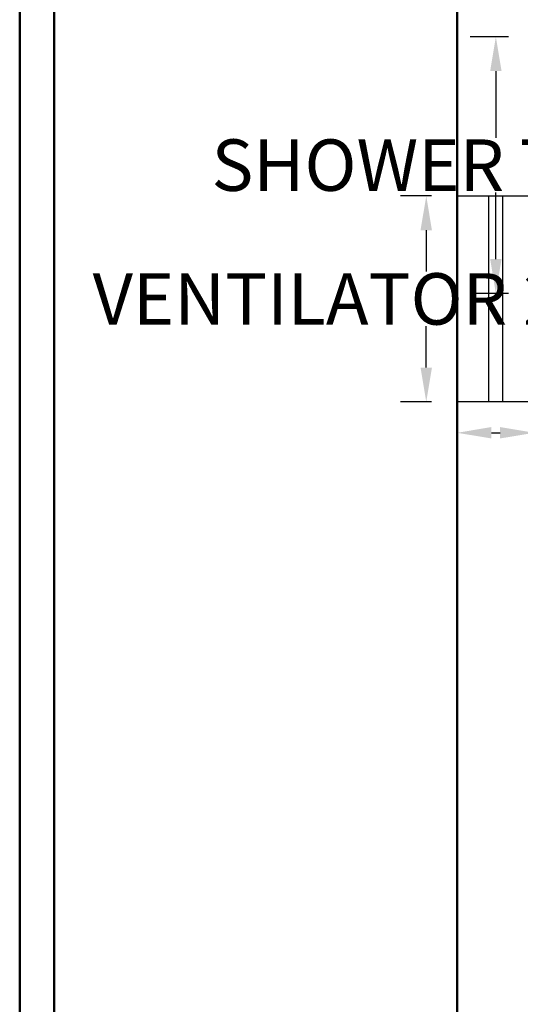
# Model space of a CAD drawing. Units: inches. Extents: x -466983 to 1020, y 324 to 318697.
# Tile 3 of 97: x 392 to 450, y 514 to 629. Entities that reach past the tile are written whole.
import ezdxf

# ---------------------------------------------------------------- set-up
doc = ezdxf.new("R2010")
doc.units = ezdxf.units.IN
doc.header["$MEASUREMENT"] = 0
for name, color, linetype, lineweight in [('A-ANNO-DIMS', 2, 'Continuous', 18), ('A-GLAZ', 4, 'Continuous', 25), ('A-WALL', 7, 'Continuous', 50)]:
    doc.layers.add(name, color=color, linetype=linetype, lineweight=lineweight)
doc.styles.get("Standard").update_dxf_attribs({"font": 'arial.ttf'})
doc.dimstyles.get("Standard").update_dxf_attribs({"dimtxt": 6, "dimasz": 4, "dimexe": 3, "dimexo": 3, "dimgap": 0.09, "dimtad": 0, "dimtih": 1, "dimtoh": 1, "dimdec": 1, "dimzin": 0, "dimdsep": 46, "dimlunit": 3, "dimtxsty": 'Standard', "dimcen": 0.09, "dimadec": 0, "dimazin": 0, "dimtfac": 1, "dimtdec": 1, "dimtofl": 0, "dimtmove": 0, "dimatfit": 3, "dimfxl": 1, "dimtolj": 1, "dimtzin": 0, "dimarcsym": 0})

# ---------------------------------------------------------------- blocks, each defined once
blk = doc.blocks.new('Ventilator')
for p, q in [((1433.59, 801.68), (1457.59, 801.68)), ((1433.59, 792.68), (1433.59, 801.68)), ((1457.59, 801.68), (1457.59, 792.68)), ((1433.59, 797.98), (1457.59, 797.98)), ((1457.59, 796.38), (1433.59, 796.38)), ((1457.59, 792.68), (1433.59, 792.68))]:
    blk.add_line(p, q)
blk = doc.blocks.new('*D61')
at = {"layer": 'A-ANNO-DIMS', "color": 0, "lineweight": -2, "transparency": 16777216}
for p, q in [((439.81, 608.4), (436.21, 608.4)), ((439.21, 604.4), (439.21, 599.6)), ((439.21, 588.4), (439.21, 593.21)), ((439.81, 584.4), (436.21, 584.4))]:
    blk.add_line(p, q, dxfattribs=at)
at = {"layer": 'A-ANNO-DIMS', "color": 0, "transparency": 16777216}
for points in [[(438.54, 604.4), (439.87, 604.4), (439.21, 608.4)], [(438.54, 588.4), (439.87, 588.4), (439.21, 584.4)]]:
    blk.add_solid(points, dxfattribs=at)
at = {"layer": 'Defpoints', "color": 0, "transparency": 16777216}
for p in [(442.81, 608.4), (439.21, 584.4), (442.81, 584.4)]:
    blk.add_point(p, dxfattribs=at)
at = {"layer": 'A-ANNO-DIMS', "color": 0, "transparency": 16777216, "insert": (439.21, 596.4), "char_height": 6, "attachment_point": 5}
blk.add_mtext('\\A1;VENTILATOR 24 TYP.', dxfattribs=at)
blk = doc.blocks.new('*D62')
at = {"layer": 'A-ANNO-DIMS', "color": 0, "lineweight": -2, "transparency": 16777216}
for p, q in [((442.81, 581.4), (442.81, 577.8)), ((446.81, 580.8), (447.81, 580.8)), ((451.81, 581.4), (451.81, 577.8)), ((451.81, 580.8), (455.81, 580.8))]:
    blk.add_line(p, q, dxfattribs=at)
at = {"layer": 'A-ANNO-DIMS', "color": 0, "transparency": 16777216}
for points in [[(446.81, 581.47), (446.81, 580.14), (442.81, 580.8)], [(447.81, 581.47), (447.81, 580.14), (451.81, 580.8)]]:
    blk.add_solid(points, dxfattribs=at)
at = {"layer": 'Defpoints', "color": 0, "transparency": 16777216}
for p in [(442.81, 584.4), (451.81, 584.4), (451.81, 580.8)]:
    blk.add_point(p, dxfattribs=at)
at = {"layer": 'A-ANNO-DIMS', "color": 0, "transparency": 16777216, "insert": (468.17, 580.8), "char_height": 6, "attachment_point": 5}
blk.add_mtext('\\A1;9 TYP.', dxfattribs=at)
blk = doc.blocks.new('*D75')
at = {"layer": 'A-ANNO-DIMS', "color": 0, "lineweight": -2, "transparency": 16777216}
for p, q in [((448.81, 626.94), (444.32, 626.94)), ((447.32, 622.94), (447.32, 615.19)), ((447.32, 601.05), (447.32, 608.8)), ((448.81, 597.05), (444.32, 597.05))]:
    blk.add_line(p, q, dxfattribs=at)
at = {"layer": 'A-ANNO-DIMS', "color": 0, "transparency": 16777216}
for points in [[(446.66, 622.94), (447.99, 622.94), (447.32, 626.94)], [(446.66, 601.05), (447.99, 601.05), (447.32, 597.05)]]:
    blk.add_solid(points, dxfattribs=at)
at = {"layer": 'Defpoints', "color": 0, "transparency": 16777216}
for p in [(451.81, 626.94), (447.32, 597.05), (451.81, 597.05)]:
    blk.add_point(p, dxfattribs=at)
at = {"layer": 'A-ANNO-DIMS', "color": 0, "transparency": 16777216, "insert": (447.32, 611.99), "char_height": 6, "attachment_point": 5}
blk.add_mtext('\\A1;SHOWER TRAY 30', dxfattribs=at)

msp = doc.modelspace()

# ---------------------------------------------------------------- linework, layer by layer
at = {"layer": 'A-WALL'}
for p, q in [((391.81, 364.94), (391.81, 1084.94)), ((442.81, 415.94), (442.81, 1084.94)), ((395.81, 368.94), (395.81, 1080.94))]:
    msp.add_line(p, q, dxfattribs=at)

# ---------------------------------------------------------------- block references
at = {"layer": 'A-GLAZ', "rotation": 270}
msp.add_blockref('Ventilator', (-349.87, 2042), dxfattribs=at)

# ---------------------------------------------------------------- dimensions: what is measured, and where the dimension line sits
at = {"layer": 'A-ANNO-DIMS'}
for base, p1, p2, text, picture, middle in [((447.32, 597.05), (451.81, 626.94), (451.81, 597.05), 'SHOWER TRAY <>', '*D75', (447.32, 611.99)), ((439.21, 584.4), (442.81, 608.4), (442.81, 584.4), 'VENTILATOR <> TYP.', '*D61', (439.21, 596.4))]:
    dim = msp.add_linear_dim(base=base, p1=p1, p2=p2, angle=270, text=text, dimstyle='Standard', override={"dimdec": 0, "dimlfac": 1, "dimrnd": 0, "dimzin": 0, "dimdsep": 46, "dimlunit": 2}, dxfattribs=at)
    dim.commit()
    dim.dimension.update_dxf_attribs({"geometry": picture, "text_midpoint": middle})
dim = msp.add_linear_dim(base=(451.81, 580.8), p1=(442.81, 584.4), p2=(451.81, 584.4), text='<> TYP.', dimstyle='Standard', override={"dimdec": 0, "dimlfac": 1, "dimrnd": 0, "dimzin": 0, "dimdsep": 46, "dimlunit": 2}, dxfattribs=at)
dim.commit()
dim.dimension.update_dxf_attribs({"geometry": '*D62', "text_midpoint": (468.17, 580.8)})

doc.saveas('drawing.dxf')
